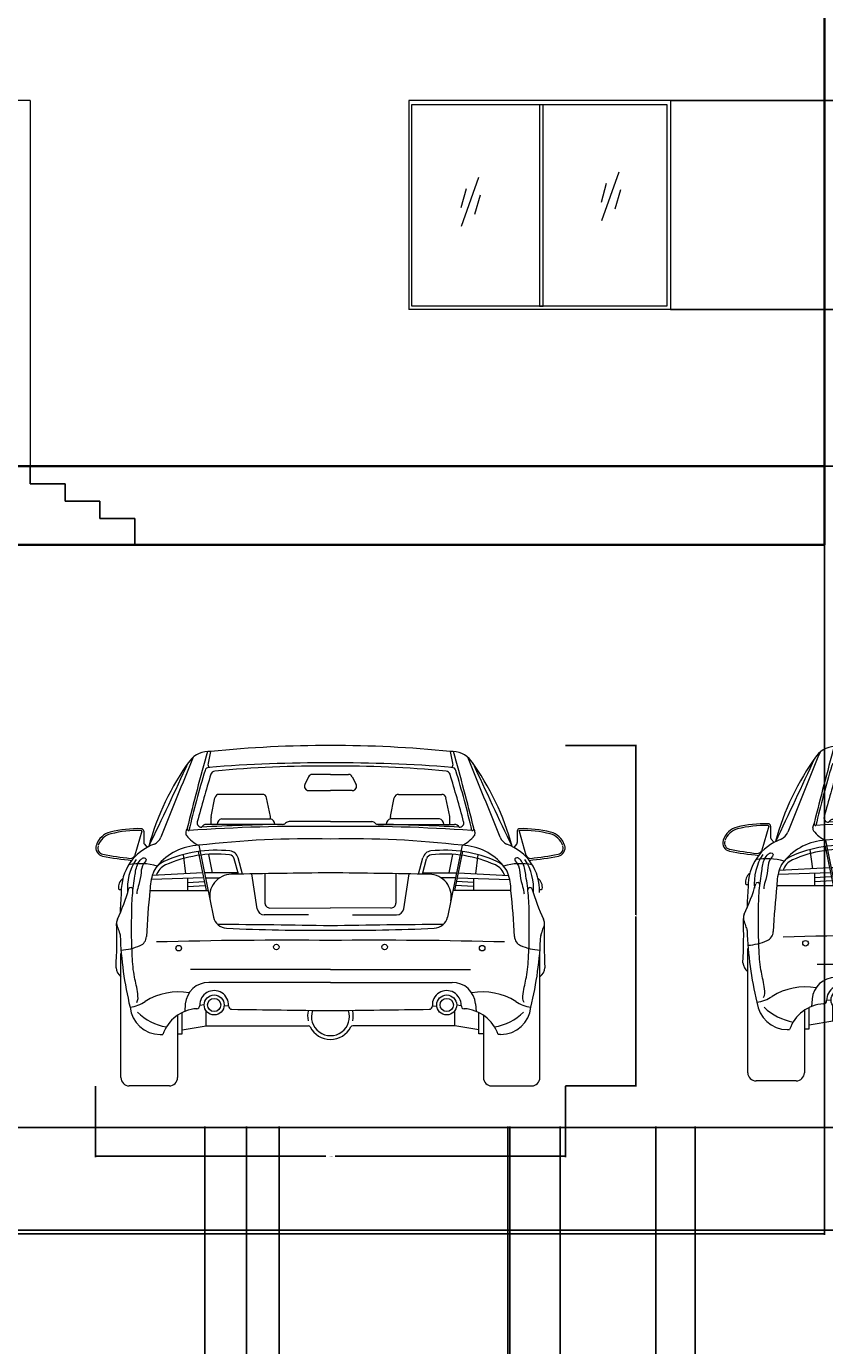
# Model space of a CAD drawing. Units: inches. Extents: x 1770 to 2988, y 1161 to 3221.
# Tile 35 of 44: x 2472 to 2655, y 2520 to 2823. Entities that reach past the tile are written whole.
import ezdxf

# ---------------------------------------------------------------- set-up
doc = ezdxf.new("R2010")
doc.units = ezdxf.units.IN
for name, color, linetype, lineweight in [('A-ANNO-DIMS', 2, 'Continuous', 18), ('A-ANNO-TTLB', 7, 'Continuous', 25), ('A-ELEV', 7, 'Continuous', 35), ('A-ELEV-DOOR', 4, 'Continuous', 18), ('A-ELEV-GLAZ', 4, 'Continuous', 18), ('A-ELEV-STRS', 7, 'Continuous', 25), ('AUDI', 8, 'Continuous', 13)]:
    doc.layers.add(name, color=color, linetype=linetype, lineweight=lineweight)
doc.styles.get("Standard").update_dxf_attribs({"font": 'arial.ttf'})
doc.dimstyles.get("Standard").update_dxf_attribs({"dimtxt": 0.18, "dimasz": 0.18, "dimexe": 0.18, "dimexo": 0.0625, "dimgap": 0.09, "dimtad": 0, "dimtih": 1, "dimtoh": 1, "dimdec": 4, "dimzin": 0, "dimdsep": 46, "dimtxsty": 'Standard', "dimcen": 0.09, "dimadec": 0, "dimazin": 0, "dimtfac": 1, "dimtdec": 4, "dimtofl": 0, "dimtmove": 0, "dimatfit": 3, "dimfxl": 1, "dimtolj": 1, "dimtzin": 0, "dimarcsym": 0})

# ---------------------------------------------------------------- blocks, each defined once
blk = doc.blocks.new('CAR-SEDAN-REAR')
for p, q in [((48.82, 70.96), (47.96, 69.22)), ((53.84, 71.5), (49.7, 71.5)), ((53.84, 71.5), (57.98, 71.5)), ((58.85, 70.96), (59.72, 69.22)), ((38.23, 66.92), (28.28, 66.92)), ((48.83, 67.81), (53.84, 67.81)), ((58.85, 67.81), (53.84, 67.81)), ((69.45, 66.92), (79.4, 66.92)), ((26.45, 61.8), (27.32, 66.14)), ((40.05, 61.84), (39.18, 66.14)), ((67.63, 61.84), (68.49, 66.14)), ((81.23, 61.8), (80.35, 66.14)), ((26.43, 60.02), (26.43, 61.6)), ((28.84, 61.32), (40.07, 61.32)), ((40.07, 61.32), (40.07, 61.65)), ((53.84, 60.68), (44.34, 60.68)), ((53.84, 60.68), (63.33, 60.68)), ((67.61, 61.32), (67.61, 61.65)), ((78.83, 61.32), (67.61, 61.32)), ((81.25, 60.02), (81.25, 61.6)), ((10.57, 58.46), (8.97, 52.97)), ((10.98, 58.46), (10.98, 55.88)), ((42.86, 60.02), (25.37, 60.02)), ((64.82, 60.02), (82.31, 60.02)), ((96.69, 58.46), (96.69, 55.88)), ((97.11, 58.46), (98.7, 52.97)), ((11.13, 55.5), (11.78, 54.75)), ((23.6, 55.23), (26.98, 38.75)), ((84.07, 55.23), (80.69, 38.75)), ((96.55, 55.5), (95.89, 54.75)), ((20.01, 53.09), (20.57, 48.7)), ((23.5, 53.8), (25.35, 44.82)), ((25.81, 53.15), (26.67, 48.92)), ((32.74, 48.6), (31.77, 52.11)), ((33.66, 48.62), (32.63, 52.35)), ((74.01, 48.62), (75.05, 52.35)), ((74.93, 48.6), (75.91, 52.11)), ((81.86, 53.15), (81, 48.92)), ((84.17, 53.8), (82.33, 44.82)), ((87.67, 53.09), (87.11, 48.7)), ((24.51, 48.92), (12.93, 48.28)), ((32.66, 48.92), (24.9, 48.92)), ((37.02, 40.63), (35.79, 48.66)), ((38.8, 48.71), (38.8, 41.97)), ((68.87, 48.71), (68.87, 41.97)), ((70.66, 40.63), (71.88, 48.66)), ((75.02, 48.92), (82.78, 48.92)), ((83.17, 48.92), (94.75, 48.28)), ((24.75, 47.73), (12.7, 47.41)), ((21.03, 47.63), (21.03, 44.82)), ((21.03, 46.7), (24.91, 46.94)), ((21.03, 45.76), (25.1, 46.01)), ((25.14, 47.73), (28.4, 47.73)), ((82.53, 47.73), (79.28, 47.73)), ((86.65, 45.76), (82.57, 46.01)), ((86.65, 46.7), (82.76, 46.94)), ((82.93, 47.73), (94.98, 47.41)), ((86.65, 47.63), (86.65, 44.82)), ((12.42, 44.82), (25.74, 44.82)), ((95.26, 44.82), (81.94, 44.82)), ((39.94, 40.83), (53.84, 40.85)), ((67.73, 40.83), (53.84, 40.85)), ((48.76, 39.24), (38.64, 39.24)), ((58.92, 39.24), (69.03, 39.24)), ((5.76, 1.88), (5.76, 30.37)), ((101.91, 1.88), (101.91, 30.37)), ((53.84, 26.71), (21.69, 26.71)), ((53.84, 26.71), (85.99, 26.71)), ((53.84, 23.76), (25.9, 23.76)), ((53.84, 23.76), (81.77, 23.76)), ((20.53, 18.8), (20.39, 17.08)), ((24.86, 18.57), (23.85, 18.45)), ((30.45, 18.32), (29.43, 18.4)), ((77.23, 18.32), (78.24, 18.4)), ((82.81, 18.57), (83.83, 18.45)), ((87.15, 18.8), (87.29, 17.08)), ((18.74, 16.2), (18.74, 1.88)), ((19.82, 11.92), (19.82, 16.83)), ((25.28, 13.8), (25.28, 17.25)), ((82.39, 13.8), (82.39, 17.25)), ((87.86, 11.92), (87.86, 16.83)), ((88.94, 16.2), (88.94, 1.88)), ((19.82, 12.84), (25.28, 13.8)), ((25.28, 13.8), (48.72, 13.8)), ((82.39, 13.8), (58.95, 13.8)), ((87.86, 12.84), (82.39, 13.8)), ((14.78, 11.78), (15.36, 11.78)), ((18.74, 11.92), (19.82, 11.92)), ((88.94, 11.92), (87.86, 11.92)), ((92.9, 11.78), (92.32, 11.78)), ((16.86, 0), (7.64, 0)), ((90.82, 0), (100.03, 0))]:
    blk.add_line(p, q)
for centre, radius in [((19.01, 31.6), 0.639), ((41.42, 31.88), 0.639), ((66.26, 31.88), 0.639), ((88.66, 31.6), 0.639), ((27.15, 18.57), 2.29), ((27.15, 18.57), 1.52), ((80.52, 18.57), 2.29), ((80.52, 18.57), 1.52)]:
    blk.add_circle(centre, radius)
for centre, radius, start, end in [((643.9, -95.37), 641.82, 164.4425, 166.06975), ((25.95, 71.16), 5.63, 85.7838, 141.6623), ((-17.33, 84), 44.29, 346.4979, 350.6005), ((54.04, -199.85), 278, 90.0409, 95.713), ((53.64, -199.85), 278, 84.287, 89.9591), ((81.73, 71.16), 5.63, 38.3377, 94.2162), ((125, 84), 44.29, 189.3995, 193.5021), ((-536.22, -95.37), 641.82, 13.93025, 15.5575), ((70.58, 39.12), 60.56, 144.0802, 164.861), ((-1004.9, 545.01), 1128.96, 334.27309, 335.34979), ((2905.78, -1097.48), 3112.89, 157.86428, 158.22937), ((26.01, 72.12), 1, 94.5001, 163.0632), ((26.15, 73.56), 0.428, 166.4979, 274.4568), ((51.95, -257.52), 331.66, 89.6747, 94.5001), ((50.83, -174.43), 247.82, 89.305, 95.4501), ((55.72, -257.52), 331.66, 85.4999, 90.3253), ((56.84, -174.43), 247.82, 84.5499, 90.695), ((81.53, 73.56), 0.428, 265.5432, 13.5021), ((81.66, 72.12), 1, 16.9368, 85.4999), ((-2798.1, -1097.48), 3112.89, 21.77063, 22.13572), ((37.09, 39.12), 60.56, 15.139, 35.9198), ((1112.58, 545.01), 1128.96, 204.65021, 205.72691), ((223.34, 12.02), 207.28, 163.0632, 167.011), ((423.22, -48.19), 414.5, 163.2127, 164.7772), ((27.39, 71.22), 1.06, 95.4501, 163.2127), ((49.7, 70.53), 0.975, 90, 153.5465), ((57.98, 70.53), 0.975, 26.4535, 90), ((80.28, 71.22), 1.06, 16.7873, 84.5499), ((-315.55, -48.19), 414.5, 15.2228, 16.7873), ((-115.67, 12.02), 207.28, 12.989, 16.9368), ((28.28, 65.95), 0.975, 90, 168.5881), ((38.23, 65.95), 0.975, 11.4119, 90), ((48.83, 68.78), 0.975, 153.5465, 270), ((58.85, 68.78), 0.975, 270, 26.4535), ((69.45, 65.95), 0.975, 90, 168.5881), ((79.4, 65.95), 0.975, 11.4119, 90), ((24.23, 60.38), 1, 164.7772, 273.0474), ((27.4, 61.6), 0.975, 168.5881, 180), ((29.25, 59.93), 1.44, 106.4998, 173.9283), ((39.09, 61.65), 0.975, 0, 11.4119), ((39.66, 59.93), 1.44, 6.0717, 73.5002), ((44.44, 59.44), 1.25, 94.4926, 135.2014), ((63.23, 59.44), 1.25, 44.7986, 85.5074), ((68.02, 59.93), 1.44, 106.4998, 173.9283), ((68.58, 61.65), 0.975, 168.5881, 180), ((78.42, 59.93), 1.44, 6.0717, 73.5002), ((80.27, 61.6), 0.975, 0, 11.4119), ((83.45, 60.38), 1, 266.9526, 15.2228), ((4.4, 53.87), 4.51, 104.0957, 161.674), ((4.4, 53.87), 4.09, 104.0957, 161.674), ((9.83, 32.25), 26.8, 88.7503, 104.0957), ((9.83, 32.25), 26.39, 88.7503, 104.0957), ((10.4, 58.46), 0.164, 0, 88.7503), ((10.4, 58.46), 0.577, 0, 88.7503), ((22.75, 57.94), 2.12, 148.8459, 175.6295), ((21.64, 58.03), 1, 175.6295, 217.0304), ((21.37, 59.04), 0.428, 166.0697, 273.9966), ((49.05, -337.24), 396.82, 89.3093, 93.9966), ((50.52, -433.5), 493.59, 90.8895, 93.0474), ((25.37, 58.77), 1.25, 90.0461, 150.7436), ((42.84, 61.02), 1, 270.8895, 315.2014), ((58.62, -337.24), 396.82, 86.0034, 90.6907), ((64.83, 61.02), 1, 224.7986, 269.1105), ((57.15, -433.5), 493.59, 86.9526, 89.1105), ((82.3, 58.77), 1.25, 29.2564, 89.9539), ((86.31, 59.04), 0.428, 266.0034, 13.9303), ((84.92, 57.94), 2.12, 4.3705, 31.1541), ((86.04, 58.03), 1, 322.9696, 4.3705), ((97.27, 58.46), 0.577, 91.2497, 180), ((97.27, 58.46), 0.164, 91.2497, 180), ((97.84, 32.25), 26.8, 75.9043, 91.2497), ((97.84, 32.25), 26.39, 75.9043, 91.2497), ((103.27, 53.87), 4.09, 18.326, 75.9043), ((103.27, 53.87), 4.51, 18.326, 75.9043), ((1.89, 54.6), 1.89, 162.3817, 258.997), ((9.28, 52.25), 9.64, 161.674, 162.3817), ((1.89, 54.6), 1.47, 162.3817, 258.997), ((17.21, 44.75), 11.38, 109.397, 181.9623), ((11.56, 55.88), 0.577, 180, 221.428), ((11.85, 58.46), 3.37, 298.1193, 335.5163), ((24.16, 42.31), 12.94, 92.4534, 141.0622), ((26.45, 61.66), 7.02, 217.0304, 246.1166), ((49.07, -161.34), 218.06, 88.7475, 96.7073), ((58.6, -161.34), 218.06, 83.2927, 91.2525), ((81.23, 61.66), 7.02, 293.8834, 322.9696), ((83.52, 42.31), 12.94, 38.9378, 87.5466), ((95.83, 58.46), 3.37, 204.4837, 241.8807), ((90.46, 44.75), 11.38, 358.0377, 70.603), ((96.12, 55.88), 0.577, 318.572, 0), ((105.79, 54.6), 1.47, 281.003, 17.6183), ((105.79, 54.6), 1.89, 281.003, 17.6183), ((98.4, 52.25), 9.64, 17.6183, 18.326), ((15.01, 122.09), 70.64, 258.997, 264.5122), ((15.01, 122.09), 70.22, 258.997, 264.1692), ((19.49, 45.28), 12.27, 146.8264, 184.9502), ((7.98, 53.25), 1.03, 264.1692, 343.8085), ((17.54, 47.23), 4.71, 114.1135, 159.9948), ((27.62, 24.7), 29.39, 83.8593, 114.1135), ((27.62, 24.7), 28.5, 83.8593, 114.1135), ((30.54, 51.77), 1.28, 15.5227, 83.8593), ((30.54, 51.77), 2.17, 15.5227, 83.8593), ((77.14, 51.77), 2.17, 96.1407, 164.4773), ((77.14, 51.77), 1.28, 96.1407, 164.4773), ((80.05, 24.7), 29.39, 65.8865, 96.1407), ((80.05, 24.7), 28.5, 65.8865, 96.1407), ((90.13, 47.23), 4.71, 20.0052, 65.8865), ((88.18, 45.28), 12.27, 355.0498, 33.1736), ((99.7, 53.25), 1.03, 196.1915, 275.8308), ((92.67, 122.09), 70.64, 275.4878, 281.003), ((92.67, 122.09), 70.22, 275.8308, 281.003), ((10.28, 37.96), 13.05, 72.9961, 102.2038), ((23.92, 44.9), 11.5, 159.9948, 180.4078), ((17.54, 47.23), 3.82, 114.1135, 163.1664), ((31.2, 43.49), 5.08, 91.0763, 191.5926), ((88.42, -3002.35), 3051.46, 90.64943, 91.0763), ((19.25, -3002.35), 3051.46, 88.9237, 89.35057), ((76.47, 43.49), 5.08, 348.4074, 88.9237), ((90.13, 47.23), 3.82, 16.8336, 65.8865), ((97.4, 37.96), 13.05, 77.7962, 107.0039), ((83.75, 44.9), 11.5, 359.5922, 20.0052), ((7.72, 45.59), 2.53, 127.0648, 188.1795), ((8.04, 45.01), 0.519, 13.0469, 148.7544), ((99.64, 45.01), 0.519, 31.2456, 166.9531), ((99.95, 45.59), 2.53, 351.8205, 52.9352), ((-40.22, 59.31), 49.83, 335.0061, 343.6424), ((5.4, 45.26), 0.184, 188.1795, 265.5447), ((5.96, 52.47), 7.42, 265.5447, 269.0559), ((86.52, 37.3), 80.99, 174.9976, 178.3487), ((182.84, 26.36), 171.42, 173.8158, 177.3495), ((-75.17, 26.36), 171.42, 2.6505, 6.1842), ((147.89, 59.31), 49.83, 196.3576, 204.9939), ((101.71, 52.47), 7.42, 270.9441, 274.4553), ((102.28, 45.26), 0.184, 274.4553, 351.8205), ((38.64, 40.88), 1.64, 188.6953, 270), ((39.94, 41.97), 1.14, 180, 270.0801), ((67.73, 41.97), 1.14, 269.9199, 0), ((69.03, 40.88), 1.64, 270, 351.3047), ((-109.4, 33.61), 114.21, 356.7448, 1.8553), ((6.82, 37.38), 2.07, 155.0061, 181.8553), ((30.15, 39.4), 3.23, 191.5926, 267.5409), ((11.27, -2447.69), 2484.8, 89.01848, 89.61606), ((96.4, -2447.69), 2484.8, 90.38394, 90.98152), ((77.52, 39.4), 3.23, 272.4591, 348.4074), ((100.86, 37.38), 2.07, 358.1447, 24.9939), ((217.07, 33.61), 114.21, 178.1447, 183.2552), ((86.52, 37.3), 80.99, 181.9837, 193.7227), ((9.23, 34.39), 2.38, 293.9425, 357.3495), ((43.39, -1053.12), 1086.55, 89.44927, 91.55649), ((51.43, 534.93), 499.22, 267.5409, 270.276), ((56.24, 534.93), 499.22, 269.724, 272.4591), ((64.28, -1053.12), 1086.55, 88.44351, 90.55073), ((98.45, 34.39), 2.38, 182.6505, 246.0575), ((21.16, 37.3), 80.99, 346.2773, 358.0163), ((5.04, 43.83), 12.7, 273.2699, 293.9425), ((102.64, 43.83), 12.7, 246.0575, 266.7301), ((7.46, 27.34), 2.84, 184.2077, 233.2585), ((100.21, 27.34), 2.84, 306.7415, 355.7923), ((18.99, 7.02), 14.55, 80.3869, 121.8355), ((25.9, 18.37), 5.39, 90, 175.3467), ((27.15, 18.57), 3.3, 356.4752, 181.7411), ((80.52, 18.57), 3.3, 358.2589, 183.5248), ((81.77, 18.37), 5.39, 4.6533, 90), ((88.69, 7.02), 14.55, 58.1645, 99.6131), ((6.88, 26.02), 7.99, 276.9357, 303.7276), ((23.11, 18.45), 0.743, 273.5063, 1.7411), ((31.19, 18.32), 0.743, 176.4752, 269.02), ((76.49, 18.32), 0.743, 270.98, 3.5248), ((84.57, 18.45), 0.743, 178.2589, 266.4937), ((100.8, 26.02), 7.99, 236.2724, 263.0643), ((14.83, 18.8), 7.02, 185.7841, 269.5996), ((18.34, 25.97), 12.64, 225.7709, 260.141), ((23.69, 8.92), 8.81, 93.5063, 161.053), ((74.78, 2566.5), 2549.29, 269.01996, 269.52932), ((53.84, 15.9), 5.24, 164.039, 190.9633), ((53.84, 15.9), 4.37, 160.8842, 19.1158), ((32.9, 2566.5), 2549.29, 270.47068, 270.98004), ((53.84, 15.9), 5.24, 349.0367, 15.961), ((83.98, 8.92), 8.81, 18.947, 86.4937), ((89.33, 25.97), 12.64, 279.859, 314.2291), ((92.85, 18.8), 7.02, 270.4004, 354.2159), ((48.72, 13.3), 0.504, 26.9755, 90), ((53.84, 15.9), 5.24, 206.9755, 333.0245), ((58.95, 13.3), 0.504, 90, 153.0245), ((7.64, 1.88), 1.88, 180, 270), ((16.86, 1.88), 1.88, 270, 0), ((90.82, 1.88), 1.88, 180, 270), ((100.03, 1.88), 1.88, 270, 0)]:
    blk.add_arc(centre, radius, start, end)
for points, knots in [([(9.37, 19.11), (9.75, 19.68), (9.62, 21.86), (8.68, 25.22), (8.18, 31.21), (8.19, 37.44), (8.27, 43.61), (8.91, 47.62), (9.28, 50.6), (10.23, 51.92), (10.94, 52.45), (11.91, 52.04), (10.48, 50.68), (10.42, 48.79), (10.02, 46.51), (9.45, 44.93), (9.41, 44.2), (9.41, 44.07)], [0, 0, 0, 0, 2.067985, 5.917661, 10.817048, 19.839487, 24.72726, 29.230389, 32.162056, 33.39317, 34.11598, 34.608356, 35.870676, 37.977272, 40.803487, 42.600574, 42.988867, 42.988867, 42.988867, 42.988867]), ([(98.31, 19.11), (97.92, 19.68), (98.06, 21.86), (98.99, 25.22), (99.49, 31.21), (99.48, 37.44), (99.4, 43.61), (98.77, 47.62), (98.4, 50.6), (97.44, 51.92), (96.74, 52.45), (95.77, 52.04), (97.19, 50.68), (97.26, 48.79), (97.66, 46.51), (98.22, 44.93), (98.26, 44.2), (98.26, 44.07)], [0, 0, 0, 0, 2.067985, 5.917661, 10.817048, 19.839487, 24.72726, 29.230389, 32.162056, 33.39317, 34.11598, 34.608356, 35.870676, 37.977272, 40.803487, 42.600574, 42.988867, 42.988867, 42.988867, 42.988867]), ([(4.75, 37.31), (4.75, 37.31), (4.77, 36.84), (5.1, 36.19), (5.34, 35.23), (5.58, 34.73), (5.58, 34.43)], [0, 0, 0, 0, 0.000002, 1.419502, 2.081106, 3.002245, 3.002245, 3.002245, 3.002245]), ([(102.92, 37.31), (102.92, 37.31), (102.9, 36.84), (102.57, 36.19), (102.33, 35.23), (102.09, 34.73), (102.09, 34.43)], [0, 0, 0, 0, 0.000002, 1.419502, 2.081106, 3.002245, 3.002245, 3.002245, 3.002245])]:
    blk.add_open_spline(points, degree=3, knots=knots)
blk = doc.blocks.new('GLASS-MARK-WINDOW')
for p, q in [((4.02, 11.23), (0.09, 0)), ((1.17, 8.59), (0, 4.27)), ((4.4, 7.13), (3.12, 2.69))]:
    blk.add_line(p, q)
blk = doc.blocks.new('*D52')
at = {"layer": 'A-ANNO-DIMS', "color": 0, "lineweight": -2, "transparency": 16777216}
for p, q in [((2488.12, 2580), (2488.12, 2563.7)), ((2595.95, 2580), (2595.95, 2563.7)), ((2488.3, 2563.88), (2540.97, 2563.88)), ((2595.77, 2563.88), (2543.1, 2563.88))]:
    blk.add_line(p, q, dxfattribs=at)
at = {"layer": 'A-ANNO-DIMS', "color": 0, "transparency": 16777216}
for points in [[(2488.3, 2563.91), (2488.3, 2563.85), (2488.12, 2563.88)], [(2595.77, 2563.91), (2595.77, 2563.85), (2595.95, 2563.88)]]:
    blk.add_solid(points, dxfattribs=at)
at = {"layer": 'Defpoints', "color": 0, "transparency": 16777216}
for p in [(2488.12, 2580.06), (2595.95, 2580.06), (2595.95, 2563.88)]:
    blk.add_point(p, dxfattribs=at)
at = {"layer": 'A-ANNO-DIMS', "color": 0, "transparency": 16777216, "insert": (2542.03, 2563.88), "char_height": 0.18, "attachment_point": 5}
blk.add_mtext('\\A1;SEDAN 108 TYP.', dxfattribs=at)
blk = doc.blocks.new('*D53')
at = {"layer": 'A-ANNO-DIMS', "color": 0, "lineweight": -2, "transparency": 16777216}
for p, q in [((2596.01, 2658.21), (2612.3, 2658.21)), ((2612.12, 2658.03), (2612.12, 2619.31)), ((2612.12, 2580.24), (2612.12, 2618.95)), ((2596.01, 2580.06), (2612.3, 2580.06))]:
    blk.add_line(p, q, dxfattribs=at)
at = {"layer": 'A-ANNO-DIMS', "color": 0, "transparency": 16777216}
for points in [[(2612.09, 2658.03), (2612.15, 2658.03), (2612.12, 2658.21)], [(2612.09, 2580.24), (2612.15, 2580.24), (2612.12, 2580.06)]]:
    blk.add_solid(points, dxfattribs=at)
at = {"layer": 'Defpoints', "color": 0, "transparency": 16777216}
for p in [(2595.95, 2658.21), (2612.12, 2658.21), (2595.95, 2580.06)]:
    blk.add_point(p, dxfattribs=at)
at = {"layer": 'A-ANNO-DIMS', "color": 0, "transparency": 16777216, "insert": (2612.12, 2619.13), "char_height": 0.18, "attachment_point": 5}
blk.add_mtext('\\A1;78 TYP.', dxfattribs=at)
blk = doc.blocks.new('*D56')
at = {"layer": 'A-ANNO-DIMS', "color": 0, "lineweight": -2, "transparency": 16777216}
for p, q in [((1971.53, 2506.34), (1971.53, 2570.7)), ((1971.71, 2570.52), (2386.59, 2570.52)), ((2802.26, 2570.52), (2387.38, 2570.52)), ((2802.44, 2506.34), (2802.44, 2570.7))]:
    blk.add_line(p, q, dxfattribs=at)
at = {"layer": 'A-ANNO-DIMS', "color": 0, "transparency": 16777216}
for points in [[(1971.71, 2570.55), (1971.71, 2570.49), (1971.53, 2570.52)], [(2802.26, 2570.55), (2802.26, 2570.49), (2802.44, 2570.52)]]:
    blk.add_solid(points, dxfattribs=at)
at = {"layer": 'Defpoints', "color": 0, "transparency": 16777216}
for p in [(2802.44, 2570.52), (1971.53, 2506.27), (2802.44, 2506.27)]:
    blk.add_point(p, dxfattribs=at)
at = {"layer": 'A-ANNO-DIMS', "color": 0, "transparency": 16777216, "insert": (2386.99, 2570.52), "char_height": 0.18, "attachment_point": 5}
blk.add_mtext('\\A1;830.9', dxfattribs=at)
blk = doc.blocks.new('*D66')
at = {"layer": 'A-ANNO-DIMS', "color": 0, "lineweight": -2, "transparency": 16777216}
for p, q in [((2397.97, 2376.76), (2397.97, 2570.7)), ((2398.15, 2570.52), (2459.91, 2570.52)), ((2522.58, 2570.52), (2460.82, 2570.52)), ((2522.76, 2376.76), (2522.76, 2570.7))]:
    blk.add_line(p, q, dxfattribs=at)
at = {"layer": 'A-ANNO-DIMS', "color": 0, "transparency": 16777216}
for points in [[(2398.15, 2570.55), (2398.15, 2570.49), (2397.97, 2570.52)], [(2522.58, 2570.55), (2522.58, 2570.49), (2522.76, 2570.52)]]:
    blk.add_solid(points, dxfattribs=at)
at = {"layer": 'Defpoints', "color": 0, "transparency": 16777216}
for p in [(2522.76, 2570.52), (2397.97, 2376.7), (2522.76, 2376.7)]:
    blk.add_point(p, dxfattribs=at)
at = {"layer": 'A-ANNO-DIMS', "color": 0, "transparency": 16777216, "insert": (2460.36, 2570.52), "char_height": 0.18, "attachment_point": 5}
blk.add_mtext('\\A1;124.78', dxfattribs=at)
blk = doc.blocks.new('*D67')
at = {"layer": 'A-ANNO-DIMS', "color": 0, "lineweight": -2, "transparency": 16777216}
for p, q in [((2582.76, 2376.76), (2582.76, 2570.7)), ((2582.94, 2570.52), (2603.83, 2570.52)), ((2625.52, 2570.52), (2604.62, 2570.52)), ((2625.7, 2376.76), (2625.7, 2570.7))]:
    blk.add_line(p, q, dxfattribs=at)
at = {"layer": 'A-ANNO-DIMS', "color": 0, "transparency": 16777216}
for points in [[(2582.94, 2570.55), (2582.94, 2570.49), (2582.76, 2570.52)], [(2625.52, 2570.55), (2625.52, 2570.49), (2625.7, 2570.52)]]:
    blk.add_solid(points, dxfattribs=at)
at = {"layer": 'Defpoints', "color": 0, "transparency": 16777216}
for p in [(2625.7, 2570.52), (2582.76, 2376.7), (2625.7, 2376.7)]:
    blk.add_point(p, dxfattribs=at)
at = {"layer": 'A-ANNO-DIMS', "color": 0, "transparency": 16777216, "insert": (2604.23, 2570.52), "char_height": 0.18, "attachment_point": 5}
blk.add_mtext('\\A1;42.94', dxfattribs=at)
blk = doc.blocks.new('*D82')
at = {"layer": 'A-ANNO-DIMS', "color": 0, "lineweight": -2, "transparency": 16777216}
for p, q in [((2443.39, 1610.26), (2443.39, 2570.7)), ((2443.57, 2570.52), (2486.45, 2570.52)), ((2530.12, 2570.52), (2487.24, 2570.52)), ((2530.3, 1610.26), (2530.3, 2570.7))]:
    blk.add_line(p, q, dxfattribs=at)
at = {"layer": 'A-ANNO-DIMS', "color": 0, "transparency": 16777216}
for points in [[(2443.57, 2570.55), (2443.57, 2570.49), (2443.39, 2570.52)], [(2530.12, 2570.55), (2530.12, 2570.49), (2530.3, 2570.52)]]:
    blk.add_solid(points, dxfattribs=at)
at = {"layer": 'Defpoints', "color": 0, "transparency": 16777216}
for p in [(2530.3, 2570.52), (2443.39, 1610.2), (2530.3, 1610.2)]:
    blk.add_point(p, dxfattribs=at)
at = {"layer": 'A-ANNO-DIMS', "color": 0, "transparency": 16777216, "insert": (2486.85, 2570.52), "char_height": 0.18, "attachment_point": 5}
blk.add_mtext('\\A1;86.92', dxfattribs=at)
blk = doc.blocks.new('*D84')
at = {"layer": 'A-ANNO-DIMS', "color": 0, "lineweight": -2, "transparency": 16777216}
for p, q in [((2513.2, 1835.26), (2513.2, 2570.7)), ((2513.38, 2570.52), (2564.56, 2570.52)), ((2616.52, 2570.52), (2565.33, 2570.52)), ((2616.7, 1835.26), (2616.7, 2570.7))]:
    blk.add_line(p, q, dxfattribs=at)
at = {"layer": 'A-ANNO-DIMS', "color": 0, "transparency": 16777216}
for points in [[(2513.38, 2570.55), (2513.38, 2570.49), (2513.2, 2570.52)], [(2616.52, 2570.55), (2616.52, 2570.49), (2616.7, 2570.52)]]:
    blk.add_solid(points, dxfattribs=at)
at = {"layer": 'Defpoints', "color": 0, "transparency": 16777216}
for p in [(2616.7, 2570.52), (2513.2, 1835.2), (2616.7, 1835.2)]:
    blk.add_point(p, dxfattribs=at)
at = {"layer": 'A-ANNO-DIMS', "color": 0, "transparency": 16777216, "insert": (2564.95, 2570.52), "char_height": 0.18, "attachment_point": 5}
blk.add_mtext('\\A1;103.5', dxfattribs=at)
blk = doc.blocks.new('*D86')
at = {"layer": 'A-ANNO-DIMS', "color": 0, "lineweight": -2, "transparency": 16777216}
for p, q in [((2583.2, 1775.21), (2583.2, 2570.7)), ((2583.38, 2570.52), (2599.62, 2570.52)), ((2616.52, 2570.52), (2600.27, 2570.52)), ((2616.7, 1775.26), (2616.7, 2570.7))]:
    blk.add_line(p, q, dxfattribs=at)
at = {"layer": 'A-ANNO-DIMS', "color": 0, "transparency": 16777216}
for points in [[(2583.38, 2570.55), (2583.38, 2570.49), (2583.2, 2570.52)], [(2616.52, 2570.55), (2616.52, 2570.49), (2616.7, 2570.52)]]:
    blk.add_solid(points, dxfattribs=at)
at = {"layer": 'Defpoints', "color": 0, "transparency": 16777216}
for p in [(2616.7, 2570.52), (2583.2, 1775.15), (2616.7, 1775.2)]:
    blk.add_point(p, dxfattribs=at)
at = {"layer": 'A-ANNO-DIMS', "color": 0, "transparency": 16777216, "insert": (2599.95, 2570.52), "char_height": 0.18, "attachment_point": 5}
blk.add_mtext('\\A1;33.5', dxfattribs=at)
blk = doc.blocks.new('*D87')
at = {"layer": 'A-ANNO-DIMS', "color": 0, "lineweight": -2, "transparency": 16777216}
for p, q in [((2594.75, 1861.4), (2594.75, 2570.7)), ((2594.93, 2570.52), (2605.33, 2570.52)), ((2616.52, 2570.52), (2606.12, 2570.52)), ((2616.7, 1839.76), (2616.7, 2570.7))]:
    blk.add_line(p, q, dxfattribs=at)
at = {"layer": 'A-ANNO-DIMS', "color": 0, "transparency": 16777216}
for points in [[(2594.93, 2570.55), (2594.93, 2570.49), (2594.75, 2570.52)], [(2616.52, 2570.55), (2616.52, 2570.49), (2616.7, 2570.52)]]:
    blk.add_solid(points, dxfattribs=at)
at = {"layer": 'Defpoints', "color": 0, "transparency": 16777216}
for p in [(2616.7, 2570.52), (2594.75, 1861.34), (2616.7, 1839.7)]:
    blk.add_point(p, dxfattribs=at)
at = {"layer": 'A-ANNO-DIMS', "color": 0, "transparency": 16777216, "insert": (2605.72, 2570.52), "char_height": 0.18, "attachment_point": 5}
blk.add_mtext('\\A1;21.95', dxfattribs=at)
blk = doc.blocks.new('*D93')
at = {"layer": 'A-ANNO-DIMS', "color": 0, "lineweight": -2, "transparency": 16777216}
for p, q in [((2181.44, 2704.23), (2181.44, 2545.88)), ((2655.44, 2704.23), (2655.44, 2545.88)), ((2181.62, 2546.06), (2418.15, 2546.06)), ((2655.26, 2546.06), (2418.74, 2546.06))]:
    blk.add_line(p, q, dxfattribs=at)
at = {"layer": 'A-ANNO-DIMS', "color": 0, "transparency": 16777216}
for points in [[(2181.62, 2546.09), (2181.62, 2546.03), (2181.44, 2546.06)], [(2655.26, 2546.09), (2655.26, 2546.03), (2655.44, 2546.06)]]:
    blk.add_solid(points, dxfattribs=at)
at = {"layer": 'Defpoints', "color": 0, "transparency": 16777216}
for p in [(2181.44, 2704.3), (2655.44, 2704.3), (2655.44, 2546.06)]:
    blk.add_point(p, dxfattribs=at)
at = {"layer": 'A-ANNO-DIMS', "color": 0, "transparency": 16777216, "insert": (2418.44, 2546.06), "char_height": 0.18, "attachment_point": 5}
blk.add_mtext('\\A1;474', dxfattribs=at)
blk = doc.blocks.new('*D96')
at = {"layer": 'A-ANNO-DIMS', "color": 0, "lineweight": -2, "transparency": 16777216}
for p, q in [((2620.11, 2758.3), (2801.91, 2758.3)), ((2801.73, 2758.12), (2801.73, 2740.48)), ((2801.73, 2722.48), (2801.73, 2740.11)), ((2655.51, 2722.3), (2801.91, 2722.3))]:
    blk.add_line(p, q, dxfattribs=at)
at = {"layer": 'A-ANNO-DIMS', "color": 0, "transparency": 16777216}
for points in [[(2801.7, 2758.12), (2801.76, 2758.12), (2801.73, 2758.3)], [(2801.7, 2722.48), (2801.76, 2722.48), (2801.73, 2722.3)]]:
    blk.add_solid(points, dxfattribs=at)
at = {"layer": 'Defpoints', "color": 0, "transparency": 16777216}
for p in [(2620.05, 2758.3), (2801.73, 2758.3), (2655.44, 2722.3)]:
    blk.add_point(p, dxfattribs=at)
at = {"layer": 'A-ANNO-DIMS', "color": 0, "transparency": 16777216, "insert": (2801.73, 2740.3), "char_height": 0.18, "attachment_point": 5}
blk.add_mtext('\\A1;36', dxfattribs=at)
blk = doc.blocks.new('*D97')
at = {"layer": 'A-ANNO-DIMS', "color": 0, "lineweight": -2, "transparency": 16777216}
for p, q in [((2620.11, 2806.3), (2801.91, 2806.3)), ((2801.73, 2806.12), (2801.73, 2782.48)), ((2801.73, 2758.48), (2801.73, 2782.11)), ((2620.11, 2758.3), (2801.91, 2758.3))]:
    blk.add_line(p, q, dxfattribs=at)
at = {"layer": 'A-ANNO-DIMS', "color": 0, "transparency": 16777216}
for points in [[(2801.7, 2806.12), (2801.76, 2806.12), (2801.73, 2806.3)], [(2801.7, 2758.48), (2801.76, 2758.48), (2801.73, 2758.3)]]:
    blk.add_solid(points, dxfattribs=at)
at = {"layer": 'Defpoints', "color": 0, "transparency": 16777216}
for p in [(2620.05, 2806.3), (2801.73, 2806.3), (2620.05, 2758.3)]:
    blk.add_point(p, dxfattribs=at)
at = {"layer": 'A-ANNO-DIMS', "color": 0, "transparency": 16777216, "insert": (2801.73, 2782.3), "char_height": 0.18, "attachment_point": 5}
blk.add_mtext('\\A1;48', dxfattribs=at)
blk = doc.blocks.new('*D98')
at = {"layer": 'A-ANNO-DIMS', "color": 0, "lineweight": -2, "transparency": 16777216}
for p, q in [((2655.51, 2842.3), (2801.91, 2842.3)), ((2801.73, 2842.12), (2801.73, 2824.48)), ((2801.73, 2806.48), (2801.73, 2824.11)), ((2620.11, 2806.3), (2801.91, 2806.3))]:
    blk.add_line(p, q, dxfattribs=at)
at = {"layer": 'A-ANNO-DIMS', "color": 0, "transparency": 16777216}
for points in [[(2801.7, 2842.12), (2801.76, 2842.12), (2801.73, 2842.3)], [(2801.7, 2806.48), (2801.76, 2806.48), (2801.73, 2806.3)]]:
    blk.add_solid(points, dxfattribs=at)
at = {"layer": 'Defpoints', "color": 0, "transparency": 16777216}
for p in [(2655.44, 2842.3), (2801.73, 2842.3), (2620.05, 2806.3)]:
    blk.add_point(p, dxfattribs=at)
at = {"layer": 'A-ANNO-DIMS', "color": 0, "transparency": 16777216, "insert": (2801.73, 2824.3), "char_height": 0.18, "attachment_point": 5}
blk.add_mtext('\\A1;36', dxfattribs=at)

msp = doc.modelspace()

# ---------------------------------------------------------------- linework, layer by layer
at = {"layer": 'A-ANNO-TTLB'}
msp.add_lwpolyline([(2073.6202, 3129.9468), (2769.3644, 3129.9468), (2769.3644, 2546.8952), (2073.6202, 2546.8952)], close=True, dxfattribs=at)
at = {"layer": 'A-ELEV'}
for p, q in [((2655.443, 2890.2969), (2655.443, 2704.2969)), ((2655.443, 2722.2969), (2181.443, 2722.2969)), ((2655.443, 2704.2969), (2181.443, 2704.2969))]:
    msp.add_line(p, q, dxfattribs=at)
at = {"layer": 'A-ELEV-DOOR'}
for q in [(2394.1592, 2806.2969), (2473.1333, 2722.2969)]:
    msp.add_line((2473.1333, 2806.2969), q, dxfattribs=at)
at = {"layer": 'A-ELEV-GLAZ'}
for p, q in [((2560.0508, 2806.2969), (2560.0508, 2758.2969)), ((2620.0508, 2806.2969), (2560.0508, 2806.2969)), ((2589.9845, 2805.3181), (2589.9845, 2759.0537)), ((2590.8648, 2759.0537), (2590.8648, 2805.3181)), ((2620.0508, 2806.2969), (2620.0508, 2758.2969)), ((2620.0508, 2758.2969), (2560.0508, 2758.2969)), ((2589.9845, 2759.0537), (2590.8648, 2759.0537))]:
    msp.add_line(p, q, dxfattribs=at)
msp.add_lwpolyline([(2560.7355, 2805.3181), (2619.2335, 2805.3181), (2619.2335, 2759.0537), (2560.7355, 2759.0537)], close=True, dxfattribs=at)
at = {"layer": 'A-ELEV-STRS'}
for p, q in [((2473.1333, 2722.2969), (2473.1333, 2718.2969)), ((2473.1333, 2718.2969), (2481.1333, 2718.2969)), ((2481.1333, 2718.2969), (2481.1333, 2714.2969)), ((2481.1333, 2714.2969), (2489.1333, 2714.2969)), ((2489.1333, 2714.2969), (2489.1333, 2710.2969)), ((2489.1333, 2710.2969), (2497.1333, 2710.2969)), ((2497.1333, 2710.2969), (2497.1333, 2704.2969))]:
    msp.add_line(p, q, dxfattribs=at)

# ---------------------------------------------------------------- block references
at = {"layer": 'A-ELEV-GLAZ'}
for p in [(2604.177, 2778.614), (2571.9757, 2777.3798)]:
    msp.add_blockref('GLASS-MARK-WINDOW', p, dxfattribs=at)
at = {"layer": 'AUDI'}
for p in [(2632.0624, 2581.1972), (2488.197, 2580.058)]:
    msp.add_blockref('CAR-SEDAN-REAR', p, dxfattribs=at)

# ---------------------------------------------------------------- dimensions: what is measured, and where the dimension line sits
at = {"layer": 'A-ANNO-DIMS'}
for base, p1, p2, picture, middle in [((2801.7346, 2842.2969), (2620.0508, 2806.2969), (2655.443, 2842.2969), '*D98', (2801.7346, 2824.2969)), ((2801.7346, 2806.2969), (2620.0508, 2758.2969), (2620.0508, 2806.2969), '*D97', (2801.7346, 2782.2969)), ((2801.7346, 2758.2969), (2655.443, 2722.2969), (2620.0508, 2758.2969), '*D96', (2801.7346, 2740.2969))]:
    dim = msp.add_linear_dim(base=base, p1=p1, p2=p2, angle=90, dimstyle='Standard', override={"dimdec": 0, "dimlfac": 1, "dimrnd": 0, "dimzin": 0, "dimdsep": 46, "dimlunit": 2}, dxfattribs=at)
    dim.commit()
    dim.dimension.update_dxf_attribs({"geometry": picture, "text_midpoint": middle})
for base, p1, p2, override, picture, middle in [((2655.443, 2546.0579), (2181.443, 2704.2969), (2655.443, 2704.2969), {"dimdec": 0, "dimlfac": 1, "dimrnd": 0, "dimzin": 0, "dimdsep": 46, "dimlunit": 2}, '*D93', (2418.443, 2546.0579)), ((2802.4374, 2570.5247), (1971.5344, 2506.2747), (2802.4374, 2506.2747), {"dimdec": 1, "dimlfac": 1, "dimrnd": 0, "dimzin": 0, "dimdsep": 46, "dimlunit": 2}, '*D56', (2386.9859, 2570.5247)), ((2522.7552, 2570.5247), (2397.9714, 2376.7021), (2522.7552, 2376.7021), {"dimdec": 2, "dimlfac": 1, "dimrnd": 0, "dimzin": 0, "dimdsep": 46, "dimlunit": 2}, '*D66', (2460.3633, 2570.5247)), ((2530.3038, 2570.5247), (2443.3863, 1610.2021), (2530.3038, 1610.2021), {"dimdec": 2, "dimlfac": 1, "dimrnd": 0, "dimzin": 0, "dimdsep": 46, "dimlunit": 2}, '*D82', (2486.8451, 2570.5247)), ((2616.696, 2570.5247), (2513.196, 1835.2021), (2616.696, 1835.2021), {"dimdec": 1, "dimlfac": 1, "dimrnd": 0, "dimzin": 0, "dimdsep": 46, "dimlunit": 2}, '*D84', (2564.946, 2570.5247)), ((2625.696, 2570.5247), (2582.7552, 2376.7021), (2625.696, 2376.7021), {"dimdec": 2, "dimlfac": 1, "dimrnd": 0, "dimzin": 0, "dimdsep": 46, "dimlunit": 2}, '*D67', (2604.2256, 2570.5247)), ((2616.696, 2570.5247), (2583.196, 1775.149), (2616.696, 1775.2021), {"dimdec": 1, "dimlfac": 1, "dimrnd": 0, "dimzin": 0, "dimdsep": 46, "dimlunit": 2}, '*D86', (2599.946, 2570.5247)), ((2616.696, 2570.5247), (2594.7479, 1861.3395), (2616.696, 1839.7021), {"dimdec": 2, "dimlfac": 1, "dimrnd": 0, "dimzin": 0, "dimdsep": 46, "dimlunit": 2}, '*D87', (2605.7219, 2570.5247))]:
    dim = msp.add_linear_dim(base=base, p1=p1, p2=p2, dimstyle='Standard', override=override, dxfattribs=at)
    dim.commit()
    dim.dimension.update_dxf_attribs({"geometry": picture, "text_midpoint": middle})
dim = msp.add_linear_dim(base=(2612.1209, 2658.2067), p1=(2595.9471, 2580.0579), p2=(2595.9471, 2658.2067), angle=90, text='<> TYP.', dimstyle='Standard', override={"dimdec": 0, "dimlfac": 1, "dimrnd": 0, "dimzin": 0, "dimdsep": 46, "dimlunit": 2}, dxfattribs=at)
dim.commit()
dim.dimension.update_dxf_attribs({"geometry": '*D53', "text_midpoint": (2612.1209, 2619.1323)})
dim = msp.add_linear_dim(base=(2595.9471, 2563.8841), p1=(2488.1224, 2580.0579), p2=(2595.9471, 2580.0579), text='SEDAN <> TYP.', dimstyle='Standard', override={"dimdec": 0, "dimlfac": 1, "dimrnd": 0, "dimzin": 0, "dimdsep": 46, "dimlunit": 2}, dxfattribs=at)
dim.commit()
dim.dimension.update_dxf_attribs({"geometry": '*D52', "text_midpoint": (2542.0348, 2563.8841)})

doc.saveas('drawing.dxf')
